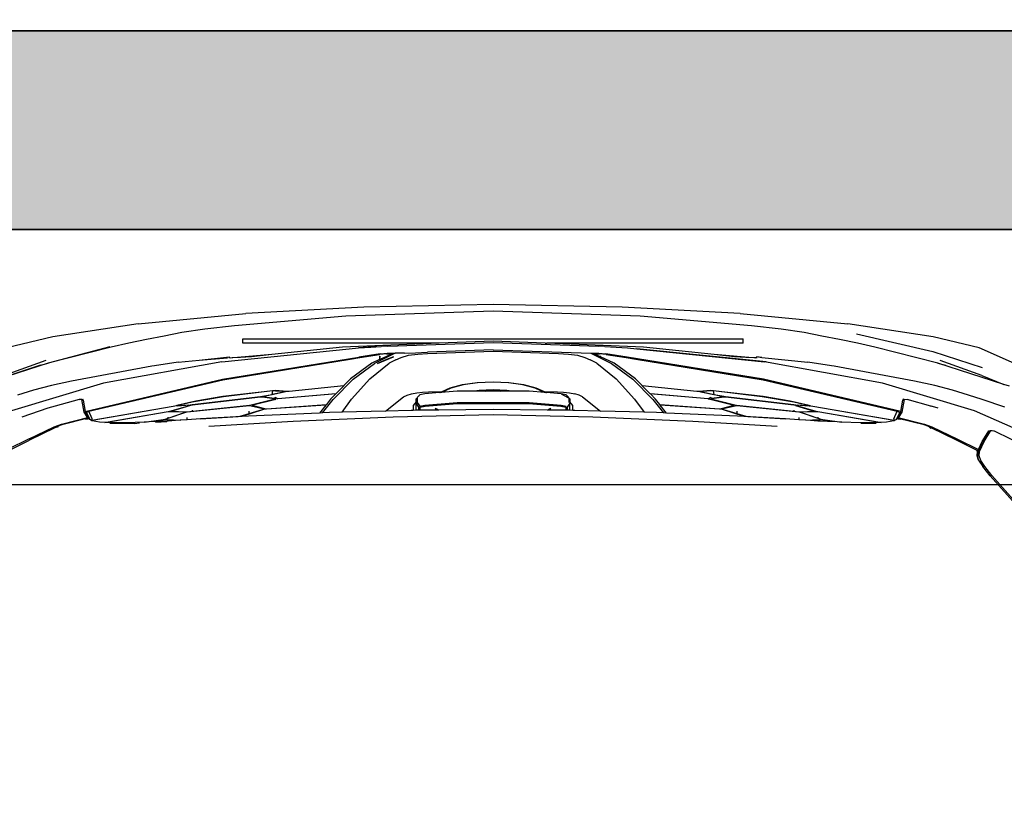
# Model space of a CAD drawing. Units: inches. Extents: x -4737294 to -4736756, y 1716389 to 1717040.
# Tile 14 of 25: x -4737171 to -4737127, y 1716633 to 1716669. Entities that reach past the tile are written whole.
import ezdxf

# ---------------------------------------------------------------- set-up
doc = ezdxf.new("R2010")
doc.units = ezdxf.units.IN
doc.header["$MEASUREMENT"] = 0
for name, color, linetype, lineweight in [('A-ANNO-DIMS', 2, 'Continuous', 18), ('A-EQPM-VEHI', 250, 'Continuous', 13), ('A-WALL-PATT', 244, 'Continuous', 13), ('walls', 252, 'Continuous', 35)]:
    doc.layers.add(name, color=color, linetype=linetype, lineweight=lineweight)
doc.layers.add('Edges', color=250, linetype='Continuous')
doc.styles.get("Standard").update_dxf_attribs({"font": 'arial.ttf'})
doc.dimstyles.get("Standard").update_dxf_attribs({"dimtxt": 8, "dimasz": 0.18, "dimexe": 0.18, "dimexo": 0.0625, "dimgap": 0.09, "dimtad": 0, "dimtih": 1, "dimtoh": 1, "dimzin": 0, "dimdsep": 46, "dimlunit": 3, "dimtxsty": 'Standard', "dimcen": 0.09, "dimadec": 0, "dimazin": 0, "dimtfac": 1, "dimtofl": 0, "dimtmove": 0, "dimatfit": 3, "dimfxl": 1, "dimtolj": 1, "dimtzin": 0, "dimarcsym": 0})

# ---------------------------------------------------------------- blocks, each defined once
blk = doc.blocks.new('Nissan Qashqai pl')
at = {"layer": 'Edges'}
for p, q in [((7.4172, 12.4431), (7.4498, 12.5093)), ((7.5369, 12.5057), (7.4635, 12.4408)), ((7.4638, 12.439), (7.5371, 12.5042)), ((7.4302, 12.4993), (7.3963, 12.4227)), ((7.347, 12.4644), (7.3309, 12.4276)), ((7.3688, 12.4532), (7.3467, 12.3846)), ((7.3596, 12.4302), (7.3688, 12.4532)), ((7.3707, 12.4592), (7.3688, 12.4532)), ((7.3925, 12.4542), (7.3845, 12.4306)), ((7.4167, 12.4393), (7.4169, 12.4406)), ((7.4167, 12.4393), (7.4172, 12.4395)), ((7.417, 12.4377), (7.4167, 12.4393)), ((7.4169, 12.4412), (7.4172, 12.4431)), ((7.4169, 12.4406), (7.4172, 12.4423)), ((7.4169, 12.4406), (7.4169, 12.4412)), ((7.4169, 12.4398), (7.4169, 12.4406)), ((7.4282, 12.4328), (7.4169, 12.4398)), ((7.4172, 12.4395), (7.4169, 12.4398)), ((7.4172, 12.4423), (7.4174, 12.4429)), ((7.4183, 12.4382), (7.4172, 12.4395)), ((7.4175, 12.4429), (7.4174, 12.4429)), ((7.4635, 12.4408), (7.4541, 12.4333)), ((7.4638, 12.439), (7.4541, 12.4313)), ((7.3345, 12.3793), (7.3514, 12.4308)), ((7.3596, 12.4302), (7.344, 12.3869)), ((7.3845, 12.4306), (7.3799, 12.4164)), ((7.4283, 12.4307), (7.417, 12.4377)), ((7.4183, 12.4382), (7.4296, 12.4312)), ((7.4387, 12.428), (7.4282, 12.4328)), ((7.4359, 12.4272), (7.4283, 12.4307)), ((7.4383, 12.4272), (7.4296, 12.4312)), ((7.4479, 12.4293), (7.4431, 12.4276)), ((7.4477, 12.427), (7.4541, 12.4313)), ((7.4541, 12.4333), (7.4479, 12.4293)), ((7.3309, 12.4276), (7.3193, 12.3797)), ((7.3963, 12.4227), (7.3676, 12.3269)), ((7.4255, 12.4044), (7.4367, 12.4268)), ((7.4365, 12.4235), (7.4267, 12.4041)), ((7.4367, 12.4268), (7.4359, 12.4272)), ((7.4378, 12.4261), (7.4365, 12.4235)), ((7.4365, 12.4235), (7.4365, 12.4235)), ((7.4367, 12.4268), (7.4383, 12.4272)), ((7.4379, 12.4263), (7.4378, 12.4261)), ((7.4379, 12.4263), (7.4383, 12.4272)), ((7.4379, 12.4263), (7.4389, 12.4269)), ((7.4384, 12.426), (7.4379, 12.4263)), ((7.4384, 12.426), (7.438, 12.4251)), ((7.4383, 12.4272), (7.4389, 12.4269)), ((7.4389, 12.4269), (7.4384, 12.426)), ((7.4387, 12.4259), (7.4384, 12.426)), ((7.4431, 12.4276), (7.4387, 12.428)), ((7.443, 12.4254), (7.4387, 12.4259)), ((7.44, 12.4264), (7.4389, 12.4269)), ((7.44, 12.4264), (7.4442, 12.4258)), ((7.4477, 12.427), (7.443, 12.4254)), ((7.4442, 12.4258), (7.4477, 12.427)), ((7.3799, 12.4164), (7.375, 12.4)), ((7.375, 12.4), (7.3699, 12.3813)), ((7.4131, 12.3783), (7.4255, 12.4044)), ((7.4267, 12.4041), (7.4139, 12.3778)), ((7.3467, 12.3846), (7.3489, 12.3925)), ((7.3193, 12.3797), (7.3059, 12.291)), ((7.3161, 12.3001), (7.3345, 12.3793)), ((7.3467, 12.3846), (7.33, 12.3192)), ((7.3699, 12.3813), (7.3653, 12.3604)), ((7.3925, 12.3813), (7.3914, 12.3775)), ((7.3937, 12.3851), (7.3925, 12.3813)), ((7.4115, 12.3746), (7.4131, 12.3783)), ((7.4139, 12.3778), (7.4122, 12.3742)), ((7.4133, 12.3759), (7.4142, 12.3776)), ((7.3913, 12.3774), (7.3844, 12.3526)), ((7.3913, 12.3774), (7.3914, 12.3775)), ((7.4033, 12.3435), (7.4101, 12.3708)), ((7.4108, 12.3703), (7.4042, 12.3435)), ((7.4101, 12.3708), (7.4115, 12.3746)), ((7.4122, 12.3742), (7.4108, 12.3703)), ((7.3653, 12.3604), (7.3497, 12.2767)), ((7.3841, 12.3485), (7.3844, 12.3526)), ((7.3846, 12.3495), (7.3841, 12.3485)), ((7.3841, 12.3485), (7.3853, 12.3483)), ((7.3846, 12.3495), (7.3976, 12.347)), ((7.3971, 12.3461), (7.3853, 12.3483)), ((7.3976, 12.347), (7.4026, 12.3439)), ((7.3971, 12.3461), (7.3635, 12.2033)), ((7.364, 12.2029), (7.3968, 12.3424)), ((7.3916, 12.2547), (7.4062, 12.3389)), ((7.4065, 12.3392), (7.3917, 12.2547)), ((7.3968, 12.3424), (7.398, 12.3449)), ((7.4046, 12.3389), (7.3968, 12.3424)), ((7.3983, 12.3458), (7.3971, 12.3461)), ((7.398, 12.3449), (7.3999, 12.344)), ((7.398, 12.3449), (7.4012, 12.3441)), ((7.4012, 12.3441), (7.3983, 12.3458)), ((7.3999, 12.344), (7.4051, 12.3415)), ((7.3999, 12.344), (7.4048, 12.3417)), ((7.4033, 12.3427), (7.4012, 12.3441)), ((7.4012, 12.3441), (7.4015, 12.344)), ((7.4015, 12.344), (7.4028, 12.3437)), ((7.4026, 12.3439), (7.4033, 12.3435)), ((7.4033, 12.3435), (7.4042, 12.3422)), ((7.4042, 12.3422), (7.4033, 12.3427)), ((7.4042, 12.3435), (7.404, 12.3429)), ((7.404, 12.3429), (7.4043, 12.3428)), ((7.404, 12.3429), (7.4043, 12.3425)), ((7.4041, 12.3435), (7.4042, 12.3435)), ((7.4042, 12.3435), (7.4045, 12.3434)), ((7.4042, 12.3422), (7.4043, 12.3425)), ((7.4044, 12.3422), (7.4042, 12.3422)), ((7.4043, 12.3428), (7.4045, 12.3434)), ((7.4043, 12.3428), (7.4046, 12.3425)), ((7.4043, 12.3425), (7.4043, 12.3428)), ((7.4043, 12.3425), (7.4044, 12.3422)), ((7.4044, 12.3422), (7.4046, 12.3419)), ((7.4046, 12.3422), (7.4044, 12.3422)), ((7.4045, 12.3434), (7.405, 12.3456)), ((7.4045, 12.3434), (7.4048, 12.3433)), ((7.4046, 12.3425), (7.4047, 12.3424)), ((7.4047, 12.3424), (7.4046, 12.3422)), ((7.4046, 12.3422), (7.4046, 12.3419)), ((7.4048, 12.3422), (7.4046, 12.3422)), ((7.4046, 12.3419), (7.405, 12.3419)), ((7.4048, 12.3417), (7.4046, 12.3419)), ((7.4046, 12.3389), (7.4062, 12.3389)), ((7.4047, 12.3424), (7.4048, 12.3422)), ((7.4048, 12.3422), (7.405, 12.3419)), ((7.4048, 12.3417), (7.4052, 12.3416)), ((7.4051, 12.3415), (7.4048, 12.3417)), ((7.405, 12.3419), (7.4052, 12.3416)), ((7.4051, 12.3415), (7.4052, 12.3415)), ((7.4052, 12.3416), (7.4052, 12.3415)), ((7.4052, 12.3415), (7.4063, 12.3395)), ((7.4062, 12.3389), (7.4063, 12.3395)), ((7.4063, 12.3395), (7.4065, 12.3392)), ((7.4065, 12.3392), (7.4066, 12.3389)), ((7.4066, 12.3389), (7.408, 12.3313)), ((7.3676, 12.3269), (7.3455, 12.2042)), ((7.408, 12.3313), (7.4083, 12.3258)), ((7.33, 12.3192), (7.3261, 12.3009)), ((7.3971, 12.2599), (7.4083, 12.3258)), ((7.4084, 12.3244), (7.3975, 12.2599)), ((7.4083, 12.3258), (7.4084, 12.3244)), ((7.4084, 12.3244), (7.4087, 12.3195)), ((7.4087, 12.3195), (7.4087, 12.3037)), ((7.4092, 12.3184), (7.4091, 12.3206)), ((7.4092, 12.305), (7.4092, 12.3184)), ((7.3261, 12.3009), (7.3223, 12.2825)), ((7.4087, 12.3037), (7.4081, 12.2848)), ((7.2951, 12.1791), (7.3059, 12.291)), ((7.3223, 12.2825), (7.3186, 12.2641)), ((7.3498, 12.2768), (7.3494, 12.2741)), ((7.3497, 12.2767), (7.3494, 12.2741)), ((7.4054, 12.2651), (7.4081, 12.2848)), ((7.4079, 12.2798), (7.4059, 12.2651)), ((7.4079, 12.2798), (7.4069, 12.2598)), ((7.4081, 12.2838), (7.4079, 12.2798)), ((7.4081, 12.2848), (7.4081, 12.2838)), ((7.3494, 12.2741), (7.3457, 12.2495)), ((7.4049, 12.2631), (7.4054, 12.2651)), ((7.4059, 12.2651), (7.4058, 12.2632)), ((7.3186, 12.2641), (7.3149, 12.2457)), ((7.3908, 12.2366), (7.3965, 12.256)), ((7.391, 12.2387), (7.3967, 12.2579)), ((7.3912, 12.2527), (7.3916, 12.2547)), ((7.3969, 12.257), (7.3965, 12.256)), ((7.3967, 12.2579), (7.3971, 12.2599)), ((7.3968, 12.2559), (7.3969, 12.257)), ((7.3972, 12.2421), (7.3968, 12.2559)), ((7.3975, 12.2599), (7.3973, 12.258)), ((7.3973, 12.258), (7.3977, 12.2439)), ((7.4048, 12.2612), (7.3982, 12.2419)), ((7.3983, 12.244), (7.4038, 12.2599)), ((7.4028, 12.2599), (7.4038, 12.2599)), ((7.4038, 12.2599), (7.4049, 12.2631)), ((7.4053, 12.2622), (7.4048, 12.2612)), ((7.4053, 12.2612), (7.4053, 12.2622)), ((7.4061, 12.2473), (7.4053, 12.2612)), ((7.4059, 12.2618), (7.4056, 12.2621)), ((7.4058, 12.2632), (7.4059, 12.2618)), ((7.4059, 12.2618), (7.4064, 12.2523)), ((7.4069, 12.2598), (7.4064, 12.2523)), ((7.3149, 12.2457), (7.3113, 12.2217)), ((7.3407, 12.2016), (7.3457, 12.2495)), ((7.3909, 12.2508), (7.3864, 12.231)), ((7.3869, 12.2347), (7.3912, 12.2527)), ((7.3901, 12.2368), (7.391, 12.2507)), ((7.3914, 12.2527), (7.3906, 12.2386)), ((7.3911, 12.2518), (7.3909, 12.2508)), ((7.391, 12.2507), (7.3911, 12.2518)), ((7.3912, 12.2517), (7.3911, 12.2518)), ((7.3917, 12.2547), (7.3914, 12.2527)), ((7.4061, 12.2472), (7.4057, 12.24)), ((7.4064, 12.2523), (7.4061, 12.2473)), ((7.4061, 12.2472), (7.4061, 12.2473)), ((7.3813, 12.2021), (7.3869, 12.2347)), ((7.3815, 12.1638), (7.3899, 12.2348)), ((7.3903, 12.2347), (7.382, 12.1639)), ((7.3899, 12.2348), (7.3901, 12.2368)), ((7.3908, 12.2366), (7.3903, 12.2347)), ((7.3905, 12.1754), (7.3966, 12.2347)), ((7.3906, 12.2386), (7.3907, 12.2376)), ((7.3907, 12.2376), (7.391, 12.2387)), ((7.3977, 12.24), (7.3911, 12.1755)), ((7.3957, 12.2348), (7.3966, 12.2348)), ((7.3957, 12.2347), (7.3966, 12.2347)), ((7.3966, 12.2348), (7.3972, 12.24)), ((7.3966, 12.2347), (7.3966, 12.2348)), ((7.3972, 12.24), (7.3972, 12.2421)), ((7.3977, 12.2439), (7.398, 12.2429)), ((7.3982, 12.2419), (7.3977, 12.24)), ((7.398, 12.2429), (7.3983, 12.244)), ((7.4032, 12.24), (7.4057, 12.24)), ((7.4057, 12.24), (7.4048, 12.2262)), ((7.3864, 12.231), (7.3815, 12.2029)), ((7.4022, 12.187), (7.4048, 12.2262)), ((7.4048, 12.2262), (7.4023, 12.1836)), ((7.3113, 12.2217), (7.3078, 12.191)), ((7.4072, 12.1299), (7.4124, 12.2176)), ((7.3455, 12.2062), (7.3317, 12.0717)), ((7.3317, 12.0717), (7.3455, 12.2042)), ((7.3407, 12.2016), (7.34, 12.1962)), ((7.34, 12.1962), (7.3401, 12.1962)), ((7.3401, 12.1962), (7.341, 12.1962)), ((7.3403, 12.1981), (7.3407, 12.2016)), ((7.3635, 12.2033), (7.3405, 12.0616)), ((7.3413, 12.1933), (7.3407, 12.1879)), ((7.341, 12.1962), (7.3414, 12.1962)), ((7.341, 12.1962), (7.341, 12.1962)), ((7.3414, 12.1962), (7.341, 12.1962)), ((7.341, 12.1962), (7.3413, 12.1933)), ((7.3415, 12.1954), (7.3413, 12.1933)), ((7.3413, 12.1933), (7.3413, 12.1931)), ((7.3426, 12.0707), (7.364, 12.2029)), ((7.375, 12.1484), (7.3813, 12.2021)), ((7.3815, 12.2029), (7.3756, 12.1509)), ((7.3078, 12.191), (7.298, 12.075)), ((7.3407, 12.1879), (7.3378, 12.1521)), ((7.341, 12.1848), (7.34, 12.1731)), ((7.3413, 12.1931), (7.341, 12.1848)), ((7.4021, 12.1833), (7.3951, 12.1606)), ((7.399, 12.1756), (7.4017, 12.185)), ((7.4017, 12.185), (7.4022, 12.187)), ((7.4023, 12.1836), (7.4018, 12.1764)), ((7.4023, 12.1836), (7.4021, 12.1833)), ((7.2951, 12.1791), (7.2884, 12.0562)), ((7.3261, 12.1821), (7.3216, 12.1821)), ((7.3216, 11.6621), (7.3216, 12.1821)), ((7.3261, 12.1821), (7.3261, 11.9779)), ((7.34, 12.1731), (7.3378, 12.1521)), ((7.3877, 12.1639), (7.3901, 12.1734)), ((7.3901, 12.1734), (7.3905, 12.1754)), ((7.3911, 12.1755), (7.3913, 12.1737)), ((7.3913, 12.1737), (7.3943, 12.1614)), ((7.3949, 12.1616), (7.399, 12.1756)), ((7.3967, 12.1756), (7.399, 12.1756)), ((7.4018, 12.1764), (7.3986, 12.1025)), ((7.3812, 12.1619), (7.3815, 12.1638)), ((7.382, 12.1639), (7.382, 12.1619)), ((7.3843, 12.1498), (7.3877, 12.1639)), ((7.3903, 12.1716), (7.3844, 12.1479)), ((7.3877, 12.1639), (7.3874, 12.1639)), ((7.3907, 12.1727), (7.3903, 12.1716)), ((7.3909, 12.1716), (7.3907, 12.1727)), ((7.3939, 12.1596), (7.3909, 12.1716)), ((7.3813, 12.1599), (7.3763, 12.1361)), ((7.3792, 12.1518), (7.3812, 12.1619)), ((7.3815, 12.161), (7.3813, 12.1599)), ((7.3817, 12.16), (7.3815, 12.161)), ((7.3832, 12.1493), (7.3817, 12.16)), ((7.382, 12.1619), (7.3838, 12.1497)), ((7.3896, 12.0954), (7.3941, 12.1576)), ((7.3945, 12.1577), (7.3903, 12.0959)), ((7.3941, 12.1576), (7.3939, 12.1596)), ((7.3943, 12.1614), (7.3947, 12.1605)), ((7.3951, 12.1606), (7.3945, 12.1577)), ((7.3947, 12.1605), (7.3949, 12.1616)), ((7.3378, 12.1521), (7.3302, 12.0785)), ((7.376, 12.136), (7.375, 12.1484)), ((7.3756, 12.1509), (7.3792, 12.1518)), ((7.3756, 12.1509), (7.3762, 12.138)), ((7.3764, 12.138), (7.3792, 12.1518)), ((7.3783, 12.0852), (7.3836, 12.1459)), ((7.384, 12.1459), (7.3788, 12.0857)), ((7.3832, 12.1493), (7.3824, 12.1487)), ((7.3824, 12.1487), (7.3832, 12.1492)), ((7.3836, 12.1459), (7.3824, 12.1487)), ((7.3824, 12.1487), (7.3835, 12.1468)), ((7.3838, 12.1497), (7.3832, 12.1493)), ((7.3832, 12.1492), (7.3837, 12.1495)), ((7.3832, 12.1492), (7.3832, 12.1493)), ((7.3836, 12.1459), (7.3835, 12.1468)), ((7.3835, 12.1468), (7.384, 12.1459)), ((7.3837, 12.1495), (7.3843, 12.1498)), ((7.3837, 12.1495), (7.3838, 12.1497)), ((7.384, 12.1459), (7.3842, 12.1495)), ((7.3844, 12.1479), (7.384, 12.1459)), ((7.3842, 12.1495), (7.3843, 12.1498)), ((7.3843, 12.1495), (7.3842, 12.1495)), ((7.3701, 12.0771), (7.3759, 12.1341)), ((7.3761, 12.1341), (7.3704, 12.0773)), ((7.3759, 12.1341), (7.376, 12.136)), ((7.3763, 12.1361), (7.3761, 12.1341)), ((7.3762, 12.137), (7.3764, 12.138)), ((7.3762, 12.138), (7.3762, 12.137)), ((7.3764, 12.1371), (7.3762, 12.137)), ((7.4025, 12.026), (7.4072, 12.1299)), ((7.3986, 12.1025), (7.3903, 12.0959)), ((7.3986, 12.1025), (7.3985, 12.0993)), ((7.3841, 12.091), (7.3788, 12.0857)), ((7.3896, 12.0954), (7.3841, 12.091)), ((7.3845, 12.0883), (7.3985, 12.0993)), ((7.3903, 12.0959), (7.3896, 12.0954)), ((7.3982, 12.092), (7.3978, 12.0791)), ((7.3985, 12.0993), (7.3982, 12.092)), ((7.3633, 12.0674), (7.3845, 12.0883)), ((7.3783, 12.0852), (7.3704, 12.0773)), ((7.3788, 12.0857), (7.3783, 12.0852)), ((7.298, 12.075), (7.2928, 11.9221)), ((7.3302, 12.0785), (7.3261, 11.9779)), ((7.3309, 12.0619), (7.3317, 12.0717)), ((7.341, 12.0605), (7.3426, 12.0707)), ((7.3701, 12.0771), (7.3631, 12.0701)), ((7.3704, 12.0773), (7.3701, 12.0771)), ((7.3842, 12.0693), (7.3978, 12.0791)), ((7.3978, 12.0791), (7.3966, 12.0338)), ((7.3294, 12.0385), (7.3309, 12.0619)), ((7.3405, 12.0616), (7.3369, 12.0394)), ((7.3377, 12.0398), (7.341, 12.0605)), ((7.3631, 12.0701), (7.3469, 12.0481)), ((7.3471, 12.0454), (7.3633, 12.0674)), ((7.363, 12.0501), (7.3842, 12.0693)), ((7.2884, 12.0562), (7.2857, 11.9221)), ((7.3468, 12.0299), (7.363, 12.0501)), ((7.3365, 12.0237), (7.3471, 12.0454)), ((7.3377, 12.0398), (7.3369, 12.0328)), ((7.3469, 12.0481), (7.3402, 12.0337)), ((7.3251, 11.9221), (7.3291, 12.0316)), ((7.3294, 12.0385), (7.3291, 12.0316)), ((7.3362, 12.0248), (7.3365, 12.0321)), ((7.3365, 12.0321), (7.3369, 12.0394)), ((7.3369, 12.0287), (7.3369, 12.0328)), ((7.3402, 12.0337), (7.338, 12.0291)), ((7.3387, 12.0332), (7.3402, 12.0337)), ((7.3468, 12.0299), (7.3432, 12.0231)), ((7.3818, 12.0151), (7.3966, 12.0338)), ((7.3966, 12.0338), (7.3959, 12.0071)), ((7.3329, 11.9221), (7.3365, 12.0237)), ((7.3362, 12.0248), (7.3366, 12.0246)), ((7.3365, 12.0237), (7.3362, 12.0248)), ((7.338, 12.0291), (7.3369, 12.0287)), ((7.3374, 12.0276), (7.3369, 12.0287)), ((7.338, 12.0291), (7.3374, 12.0276)), ((7.3407, 12.0176), (7.3432, 12.0231)), ((7.4002, 11.9221), (7.4025, 12.026)), ((7.3373, 12.0004), (7.3386, 12.01)), ((7.3386, 12.01), (7.3407, 12.0176)), ((7.3801, 12.0115), (7.3786, 12.007)), ((7.3818, 12.0151), (7.3801, 12.0115)), ((7.3367, 11.99), (7.3373, 12.0004)), ((7.3768, 11.9954), (7.3775, 12.0015)), ((7.3775, 12.0015), (7.3786, 12.007)), ((7.3808, 11.9993), (7.3798, 11.9983)), ((7.3807, 11.9991), (7.3798, 11.9983)), ((7.38, 11.9953), (7.383, 12.0011)), ((7.3807, 11.9991), (7.3808, 11.9993)), ((7.381, 11.9993), (7.3807, 11.9991)), ((7.3808, 11.9993), (7.384, 12.0021)), ((7.381, 11.9993), (7.3808, 11.9993)), ((7.383, 12.0011), (7.381, 11.9993)), ((7.3866, 12.0011), (7.383, 12.0011)), ((7.384, 12.0021), (7.387, 12.0021)), ((7.3868, 12.002), (7.3866, 12.0011)), ((7.3875, 12.0011), (7.3866, 12.0011)), ((7.387, 12.0021), (7.3868, 12.002)), ((7.3909, 12.0051), (7.387, 12.0021)), ((7.387, 12.0021), (7.3885, 12.0021)), ((7.3885, 12.0021), (7.3925, 11.9993)), ((7.3955, 12.0021), (7.3885, 12.0021)), ((7.3956, 12.0051), (7.3909, 12.0051)), ((7.3925, 11.9993), (7.3958, 11.9993)), ((7.3925, 11.9993), (7.3929, 11.9981)), ((7.3955, 12.0021), (7.3958, 12.0018)), ((7.3959, 12.0049), (7.3956, 12.0051)), ((7.3959, 12.0051), (7.3956, 12.0051)), ((7.3959, 12.0049), (7.3958, 12.0018)), ((7.3958, 12.0018), (7.3958, 11.9993)), ((7.3958, 11.9993), (7.3958, 11.9981)), ((7.3959, 12.0071), (7.3959, 12.0051)), ((7.3959, 12.0051), (7.3959, 12.0049)), ((7.3343, 11.9221), (7.3367, 11.99)), ((7.3761, 11.9751), (7.3765, 11.989)), ((7.3765, 11.989), (7.3768, 11.9954)), ((7.3787, 11.9928), (7.3774, 11.9778)), ((7.3798, 11.9983), (7.3787, 11.9928)), ((7.3787, 11.9928), (7.38, 11.9953)), ((7.3876, 11.9595), (7.3904, 11.9928)), ((7.3917, 11.9926), (7.3889, 11.9594)), ((7.3904, 11.9928), (7.3916, 11.9983)), ((7.3929, 11.9981), (7.3917, 11.9926)), ((7.3958, 11.9981), (7.3929, 11.9981)), ((7.3958, 11.9981), (7.3956, 11.9801)), ((7.3938, 11.9823), (7.3956, 11.9801)), ((7.3956, 11.9788), (7.3938, 11.981)), ((7.3956, 11.9788), (7.3951, 11.9221)), ((7.3956, 11.9801), (7.3956, 11.9788)), ((7.3261, 11.9764), (7.3238, 11.9221)), ((7.3261, 11.9764), (7.3261, 11.9779)), ((7.3724, 11.9667), (7.3761, 11.9751)), ((7.3771, 11.9757), (7.3727, 11.9658)), ((7.3773, 11.9759), (7.3759, 11.9595)), ((7.3761, 11.9751), (7.3769, 11.9767)), ((7.3769, 11.9767), (7.3771, 11.977)), ((7.3774, 11.9778), (7.3771, 11.9771)), ((7.3771, 11.9771), (7.3774, 11.9774)), ((7.3771, 11.9771), (7.3771, 11.977)), ((7.3773, 11.9759), (7.3771, 11.9757)), ((7.3774, 11.9774), (7.3773, 11.9759)), ((7.3774, 11.9774), (7.3774, 11.9778)), ((7.369, 11.9536), (7.3724, 11.9667)), ((7.3727, 11.9658), (7.3693, 11.953)), ((7.3759, 11.9595), (7.3759, 11.9417)), ((7.3876, 11.8847), (7.3876, 11.9595)), ((7.3889, 11.9594), (7.3889, 11.8848)), ((7.3668, 11.9384), (7.369, 11.9536)), ((7.3693, 11.953), (7.3672, 11.9381)), ((7.3661, 11.9221), (7.3668, 11.9384)), ((7.3672, 11.9381), (7.3665, 11.9221)), ((7.3759, 11.9417), (7.3751, 11.9363)), ((7.3759, 11.9417), (7.3759, 11.9303)), ((7.3751, 11.9363), (7.3745, 11.9221)), ((7.3755, 11.9221), (7.3759, 11.9303)), ((7.3759, 11.9303), (7.3759, 11.9139)), ((7.2857, 11.9221), (7.2884, 11.7879)), ((7.2928, 11.9221), (7.298, 11.7692)), ((7.3238, 11.9221), (7.3261, 11.8662)), ((7.3291, 11.8126), (7.3251, 11.9221)), ((7.3329, 11.9221), (7.3354, 11.8539)), ((7.3367, 11.8541), (7.3343, 11.9221)), ((7.3668, 11.9057), (7.3661, 11.9221)), ((7.3665, 11.9221), (7.3672, 11.9061)), ((7.3745, 11.9221), (7.3751, 11.9078)), ((7.3759, 11.9139), (7.3755, 11.9221)), ((7.3951, 11.9221), (7.3956, 11.8653)), ((7.4025, 11.8181), (7.4002, 11.9221)), ((7.3751, 11.9078), (7.3759, 11.9025)), ((7.3759, 11.9139), (7.3759, 11.9025)), ((7.369, 11.8905), (7.3668, 11.9057)), ((7.3672, 11.9061), (7.3693, 11.8911)), ((7.3759, 11.9025), (7.3759, 11.8847)), ((7.3724, 11.8775), (7.369, 11.8905)), ((7.3693, 11.8911), (7.3727, 11.8783)), ((7.3761, 11.8691), (7.3724, 11.8775)), ((7.3727, 11.8783), (7.3771, 11.8685)), ((7.3759, 11.8847), (7.3773, 11.8682)), ((7.3904, 11.8513), (7.3876, 11.8847)), ((7.3889, 11.8848), (7.3917, 11.8516)), ((7.3261, 11.8662), (7.3302, 11.7656)), ((7.3261, 11.8662), (7.3261, 11.6621)), ((7.3765, 11.8551), (7.3761, 11.8691)), ((7.3769, 11.8674), (7.3761, 11.8691)), ((7.3771, 11.8671), (7.3769, 11.8674)), ((7.3771, 11.8685), (7.3773, 11.8682)), ((7.3771, 11.8671), (7.3771, 11.8671)), ((7.3771, 11.8671), (7.3774, 11.8664)), ((7.3774, 11.8668), (7.3771, 11.8671)), ((7.3773, 11.8682), (7.3774, 11.8668)), ((7.3774, 11.8668), (7.3774, 11.8664)), ((7.3774, 11.8664), (7.3787, 11.8513)), ((7.3938, 11.8632), (7.3956, 11.8653)), ((7.3956, 11.864), (7.3938, 11.8619)), ((7.3956, 11.8653), (7.3956, 11.864)), ((7.3956, 11.864), (7.3958, 11.8461)), ((7.3361, 11.8416), (7.3354, 11.8539)), ((7.3373, 11.8438), (7.3367, 11.8541)), ((7.3768, 11.8488), (7.3765, 11.8551)), ((7.3775, 11.8427), (7.3768, 11.8488)), ((7.3787, 11.8513), (7.3798, 11.8459)), ((7.3798, 11.8459), (7.3808, 11.8448)), ((7.3875, 11.8431), (7.3916, 11.8459)), ((7.3916, 11.8459), (7.3904, 11.8513)), ((7.3917, 11.8516), (7.3929, 11.8461)), ((7.3929, 11.8461), (7.3925, 11.8448)), ((7.3929, 11.8461), (7.3958, 11.8461)), ((7.3958, 11.8461), (7.3958, 11.8448)), ((7.3362, 11.8301), (7.3361, 11.8416)), ((7.3386, 11.8342), (7.3373, 11.8438)), ((7.3786, 11.8372), (7.3775, 11.8427)), ((7.3801, 11.8327), (7.3786, 11.8372)), ((7.3808, 11.8448), (7.3807, 11.8451)), ((7.3808, 11.8448), (7.381, 11.8448)), ((7.384, 11.8421), (7.3808, 11.8448)), ((7.383, 11.8431), (7.3875, 11.8431)), ((7.387, 11.8421), (7.384, 11.8421)), ((7.387, 11.8421), (7.3909, 11.8391)), ((7.3885, 11.8421), (7.387, 11.8421)), ((7.3925, 11.8448), (7.3885, 11.8421)), ((7.3955, 11.8421), (7.3885, 11.8421)), ((7.3909, 11.8391), (7.3956, 11.8391)), ((7.3958, 11.8448), (7.3925, 11.8448)), ((7.3958, 11.8423), (7.3955, 11.8421)), ((7.3956, 11.8391), (7.3959, 11.8392)), ((7.3956, 11.8391), (7.3959, 11.8391)), ((7.3958, 11.8448), (7.3958, 11.8423)), ((7.3958, 11.8423), (7.3959, 11.8392)), ((7.3959, 11.8392), (7.3959, 11.8391)), ((7.3959, 11.8391), (7.3959, 11.8371)), ((7.3959, 11.8371), (7.3966, 11.8103)), ((7.3362, 11.8301), (7.3365, 11.8204)), ((7.3407, 11.8266), (7.3386, 11.8342)), ((7.3432, 11.821), (7.3407, 11.8266)), ((7.3818, 11.8291), (7.3801, 11.8327)), ((7.3966, 11.8103), (7.3818, 11.8291)), ((7.3362, 11.8194), (7.3365, 11.8204)), ((7.3367, 11.8196), (7.3362, 11.8194)), ((7.3365, 11.812), (7.3362, 11.8194)), ((7.3365, 11.8204), (7.3471, 11.7987)), ((7.3369, 11.8155), (7.3374, 11.8165)), ((7.3369, 11.8113), (7.3369, 11.8155)), ((7.3369, 11.8155), (7.338, 11.8151)), ((7.3374, 11.8165), (7.338, 11.8151)), ((7.338, 11.8151), (7.343, 11.8045)), ((7.3401, 11.8186), (7.3431, 11.8112)), ((7.347, 11.8021), (7.3401, 11.8186)), ((7.3432, 11.821), (7.3468, 11.8142)), ((7.4072, 11.7142), (7.4025, 11.8181)), ((7.3291, 11.8126), (7.3294, 11.8057)), ((7.3301, 11.7949), (7.3294, 11.8057)), ((7.3369, 11.8047), (7.3365, 11.812)), ((7.3369, 11.8113), (7.3377, 11.8044)), ((7.3369, 11.8047), (7.3405, 11.7825)), ((7.3377, 11.8042), (7.3377, 11.8044)), ((7.343, 11.8045), (7.3396, 11.8043)), ((7.3396, 11.8043), (7.3431, 11.8042)), ((7.343, 11.8045), (7.3431, 11.8042)), ((7.3431, 11.8112), (7.347, 11.8021)), ((7.363, 11.794), (7.3468, 11.8142)), ((7.3966, 11.8103), (7.3978, 11.7651)), ((7.3295, 11.8012), (7.3309, 11.7822)), ((7.3295, 11.8012), (7.3301, 11.7949)), ((7.3309, 11.7822), (7.3301, 11.7949)), ((7.341, 11.7837), (7.3377, 11.8042)), ((7.3431, 11.8042), (7.3469, 11.7961)), ((7.3469, 11.7961), (7.3631, 11.774)), ((7.3633, 11.7767), (7.3471, 11.7987)), ((7.3842, 11.7749), (7.363, 11.794)), ((7.2884, 11.7879), (7.2951, 11.6651)), ((7.3317, 11.7724), (7.3309, 11.7822)), ((7.3635, 11.6409), (7.3405, 11.7825)), ((7.3426, 11.7735), (7.341, 11.7837)), ((7.3631, 11.774), (7.3701, 11.7671)), ((7.3845, 11.7558), (7.3633, 11.7767)), ((7.3978, 11.7651), (7.3842, 11.7749)), ((7.298, 11.7692), (7.3078, 11.6532)), ((7.3302, 11.7656), (7.3378, 11.6921)), ((7.3455, 11.64), (7.3317, 11.7724)), ((7.364, 11.6413), (7.3426, 11.7735)), ((7.3759, 11.7101), (7.3701, 11.7671)), ((7.3701, 11.7671), (7.3704, 11.7668)), ((7.3704, 11.7668), (7.3761, 11.71)), ((7.3704, 11.7668), (7.3783, 11.759)), ((7.3978, 11.7651), (7.3982, 11.7521)), ((7.3836, 11.6983), (7.3783, 11.759)), ((7.3783, 11.759), (7.3788, 11.7585)), ((7.3788, 11.7585), (7.384, 11.6982)), ((7.3788, 11.7585), (7.3841, 11.7532)), ((7.3841, 11.7532), (7.3896, 11.7488)), ((7.3985, 11.7448), (7.3845, 11.7558)), ((7.3941, 11.6865), (7.3896, 11.7488)), ((7.3896, 11.7488), (7.3903, 11.7483)), ((7.3903, 11.7483), (7.3945, 11.6865)), ((7.3903, 11.7483), (7.3986, 11.7417)), ((7.3982, 11.7521), (7.3985, 11.7448)), ((7.3985, 11.7448), (7.3986, 11.7417)), ((7.3986, 11.7417), (7.4018, 11.6678)), ((7.4124, 11.6265), (7.4072, 11.7142)), ((7.375, 11.6957), (7.376, 11.7081)), ((7.3762, 11.7062), (7.3757, 11.6959)), ((7.376, 11.7081), (7.3759, 11.7101)), ((7.3761, 11.71), (7.3763, 11.7081)), ((7.3762, 11.7062), (7.3764, 11.7061)), ((7.3763, 11.7081), (7.3813, 11.6842)), ((7.3764, 11.7061), (7.3792, 11.6924)), ((7.3378, 11.6921), (7.3407, 11.6563)), ((7.3378, 11.6921), (7.34, 11.671)), ((7.3813, 11.642), (7.375, 11.6957)), ((7.3757, 11.6959), (7.3756, 11.6933)), ((7.3792, 11.6924), (7.3756, 11.6933)), ((7.3756, 11.6933), (7.3815, 11.6413)), ((7.3757, 11.6959), (7.3757, 11.6959)), ((7.3812, 11.6823), (7.3792, 11.6924)), ((7.3817, 11.6844), (7.3832, 11.6949)), ((7.3838, 11.6944), (7.382, 11.6823)), ((7.3824, 11.6955), (7.3836, 11.6983)), ((7.3835, 11.6973), (7.3824, 11.6955)), ((7.3834, 11.6959), (7.3824, 11.6955)), ((7.3824, 11.6955), (7.3832, 11.6949)), ((7.3832, 11.695), (7.3824, 11.6955)), ((7.3832, 11.695), (7.3834, 11.6959)), ((7.3838, 11.6947), (7.3832, 11.695)), ((7.3832, 11.6949), (7.3838, 11.6944)), ((7.3837, 11.696), (7.3834, 11.6959)), ((7.3835, 11.6973), (7.3836, 11.6983)), ((7.3836, 11.6975), (7.3835, 11.6973)), ((7.3836, 11.6975), (7.3836, 11.6983)), ((7.384, 11.6982), (7.3836, 11.6975)), ((7.3844, 11.6963), (7.3837, 11.696)), ((7.3838, 11.6947), (7.3837, 11.696)), ((7.3843, 11.6944), (7.3838, 11.6947)), ((7.3843, 11.6942), (7.3838, 11.6944)), ((7.3843, 11.6944), (7.3844, 11.6963)), ((7.3843, 11.6942), (7.3843, 11.6944)), ((7.3877, 11.6803), (7.3843, 11.6942)), ((7.3844, 11.6963), (7.3903, 11.6725)), ((7.3815, 11.6804), (7.3812, 11.6823)), ((7.3813, 11.6842), (7.3817, 11.6844)), ((7.3817, 11.6841), (7.3813, 11.6842)), ((7.3817, 11.6841), (7.3817, 11.6844)), ((7.382, 11.6823), (7.382, 11.6803)), ((7.3909, 11.6728), (7.3939, 11.6846)), ((7.3943, 11.6827), (7.3913, 11.6705)), ((7.3939, 11.6846), (7.3941, 11.6865)), ((7.3943, 11.6827), (7.3949, 11.6826)), ((7.3943, 11.6827), (7.395, 11.6825)), ((7.3945, 11.6865), (7.3951, 11.6835)), ((7.395, 11.6825), (7.3949, 11.6826)), ((7.399, 11.6686), (7.395, 11.6825)), ((7.3951, 11.6835), (7.4021, 11.6609)), ((7.3899, 11.6094), (7.3815, 11.6804)), ((7.382, 11.6803), (7.3903, 11.6095)), ((7.3874, 11.6803), (7.3877, 11.6803)), ((7.3901, 11.6707), (7.3877, 11.6803)), ((7.3909, 11.6728), (7.3903, 11.6725)), ((7.3909, 11.6725), (7.3903, 11.6725)), ((7.3909, 11.6725), (7.3909, 11.6728)), ((7.3059, 11.5532), (7.2951, 11.6651)), ((7.3261, 11.6621), (7.3216, 11.6621)), ((7.34, 11.671), (7.341, 11.6594)), ((7.3905, 11.6687), (7.3901, 11.6707)), ((7.3966, 11.6095), (7.3905, 11.6687)), ((7.3913, 11.6705), (7.3911, 11.6687)), ((7.3911, 11.6687), (7.3977, 11.6042)), ((7.399, 11.6686), (7.3967, 11.6686)), ((7.4017, 11.6592), (7.399, 11.6686)), ((7.4018, 11.6678), (7.4022, 11.6609)), ((7.4022, 11.6609), (7.4021, 11.6609)), ((7.4022, 11.6609), (7.4022, 11.6609)), ((7.3078, 11.6532), (7.3113, 11.6224)), ((7.3407, 11.6563), (7.3413, 11.6509)), ((7.341, 11.6594), (7.3413, 11.6511)), ((7.341, 11.648), (7.3413, 11.6509)), ((7.3413, 11.6511), (7.3413, 11.6509)), ((7.3413, 11.6509), (7.3415, 11.6488)), ((7.4022, 11.6571), (7.4017, 11.6592)), ((7.4022, 11.6609), (7.4021, 11.6609)), ((7.4022, 11.6609), (7.4048, 11.618)), ((7.4048, 11.618), (7.4022, 11.6571)), ((7.3401, 11.648), (7.34, 11.648)), ((7.3438, 11.6167), (7.34, 11.648)), ((7.341, 11.648), (7.3401, 11.648)), ((7.3414, 11.648), (7.341, 11.648)), ((7.341, 11.648), (7.3414, 11.648)), ((7.3438, 11.6167), (7.3412, 11.646)), ((7.3971, 11.4981), (7.3635, 11.6409)), ((7.3968, 11.5018), (7.364, 11.6413)), ((7.3869, 11.6094), (7.3813, 11.642)), ((7.3815, 11.6413), (7.3864, 11.6131)), ((7.3455, 11.64), (7.3676, 11.5172)), ((7.3113, 11.6224), (7.3149, 11.5984)), ((7.3457, 11.5947), (7.3438, 11.6167)), ((7.3864, 11.6131), (7.3909, 11.5933)), ((7.4048, 11.618), (7.4057, 11.6042)), ((7.3912, 11.5914), (7.3869, 11.6094)), ((7.3901, 11.6073), (7.3899, 11.6094)), ((7.391, 11.5935), (7.3901, 11.6073)), ((7.3903, 11.6095), (7.3908, 11.6076)), ((7.3906, 11.6055), (7.391, 11.6055)), ((7.3906, 11.6055), (7.391, 11.6054)), ((7.3906, 11.6055), (7.3914, 11.5914)), ((7.3908, 11.6076), (7.3965, 11.5881)), ((7.391, 11.6054), (7.391, 11.6055)), ((7.3967, 11.5862), (7.391, 11.6054)), ((7.3966, 11.6095), (7.3957, 11.6095)), ((7.3972, 11.6042), (7.3966, 11.6095)), ((7.3968, 11.5882), (7.3972, 11.6021)), ((7.3972, 11.6021), (7.3972, 11.6042)), ((7.3977, 11.6003), (7.3973, 11.5862)), ((7.3977, 11.6042), (7.3982, 11.6022)), ((7.3977, 11.6003), (7.3983, 11.6002)), ((7.3977, 11.6003), (7.3983, 11.6001)), ((7.3982, 11.6022), (7.4048, 11.5829)), ((7.3983, 11.6001), (7.3983, 11.6002)), ((7.4038, 11.5843), (7.3983, 11.6001)), ((7.4057, 11.6042), (7.4032, 11.6042)), ((7.4057, 11.6042), (7.4061, 11.597)), ((7.3149, 11.5984), (7.3186, 11.58)), ((7.3457, 11.5947), (7.3494, 11.57)), ((7.391, 11.5935), (7.3909, 11.5933)), ((7.391, 11.5934), (7.3909, 11.5933)), ((7.3916, 11.5894), (7.3912, 11.5914)), ((7.3914, 11.5914), (7.3917, 11.5895)), ((7.4062, 11.5053), (7.3916, 11.5894)), ((7.3917, 11.5895), (7.4065, 11.505)), ((7.4053, 11.5831), (7.4061, 11.5969)), ((7.4064, 11.5919), (7.406, 11.5834)), ((7.4061, 11.5969), (7.4061, 11.597)), ((7.4061, 11.5969), (7.4064, 11.5919)), ((7.4064, 11.5919), (7.4069, 11.5844)), ((7.3186, 11.58), (7.3223, 11.5616)), ((7.3968, 11.5882), (7.3965, 11.5881)), ((7.3971, 11.5842), (7.3967, 11.5862)), ((7.3968, 11.5882), (7.3973, 11.5884)), ((7.4083, 11.5184), (7.3971, 11.5842)), ((7.3973, 11.5862), (7.3975, 11.5843)), ((7.3975, 11.5843), (7.4084, 11.5198)), ((7.4038, 11.5843), (7.4028, 11.5843)), ((7.4049, 11.5811), (7.4038, 11.5843)), ((7.4053, 11.5831), (7.4048, 11.5829)), ((7.4053, 11.583), (7.4048, 11.5829)), ((7.4054, 11.5791), (7.4049, 11.5811)), ((7.406, 11.5834), (7.4053, 11.5831)), ((7.406, 11.5833), (7.4053, 11.583)), ((7.4053, 11.583), (7.4053, 11.5831)), ((7.4081, 11.5593), (7.4054, 11.5791)), ((7.406, 11.5833), (7.4058, 11.581)), ((7.4058, 11.581), (7.4059, 11.579)), ((7.4059, 11.579), (7.4079, 11.5644)), ((7.406, 11.5834), (7.406, 11.5833)), ((7.4069, 11.5844), (7.4079, 11.5644)), ((7.4081, 11.5711), (7.4075, 11.5828)), ((7.3494, 11.57), (7.3497, 11.5674)), ((7.3494, 11.57), (7.3498, 11.5674)), ((7.3223, 11.5616), (7.3261, 11.5433)), ((7.3497, 11.5674), (7.3653, 11.4838)), ((7.4079, 11.5644), (7.4081, 11.5604)), ((7.4079, 11.5644), (7.4081, 11.5629)), ((7.4081, 11.5604), (7.4081, 11.5593)), ((7.4081, 11.5593), (7.4087, 11.5405)), ((7.3059, 11.5532), (7.3193, 11.4645)), ((7.4092, 11.5416), (7.409, 11.5485)), ((7.4096, 11.549), (7.4092, 11.5521)), ((7.4093, 11.5546), (7.4095, 11.5529)), ((7.3261, 11.5433), (7.33, 11.5249)), ((7.4087, 11.5405), (7.4087, 11.5246)), ((7.4092, 11.5258), (7.4092, 11.5416)), ((7.3297, 11.5237), (7.3467, 11.4596)), ((7.33, 11.5249), (7.3467, 11.4596)), ((7.4083, 11.5184), (7.408, 11.5129)), ((7.4084, 11.5198), (7.4083, 11.5184)), ((7.4087, 11.5246), (7.4084, 11.5198)), ((7.4091, 11.5235), (7.4092, 11.5258)), ((7.3676, 11.5172), (7.3963, 11.4215)), ((7.408, 11.5129), (7.4066, 11.5052)), ((7.3976, 11.4971), (7.3846, 11.4946)), ((7.3853, 11.4958), (7.3971, 11.4981)), ((7.4046, 11.5053), (7.3968, 11.5018)), ((7.398, 11.4993), (7.3968, 11.5018)), ((7.3971, 11.4981), (7.3983, 11.4983)), ((7.4026, 11.5002), (7.3976, 11.4971)), ((7.398, 11.4993), (7.4048, 11.5024)), ((7.4012, 11.5001), (7.398, 11.4993)), ((7.3983, 11.4983), (7.4012, 11.5001)), ((7.4012, 11.5001), (7.4033, 11.5014)), ((7.403, 11.5005), (7.4026, 11.5002)), ((7.403, 11.5005), (7.4028, 11.5004)), ((7.4033, 11.5007), (7.403, 11.5005)), ((7.4033, 11.5014), (7.4042, 11.502)), ((7.4042, 11.502), (7.4033, 11.5007)), ((7.4033, 11.5005), (7.4033, 11.5007)), ((7.4034, 11.5005), (7.4033, 11.5005)), ((7.4101, 11.4733), (7.4033, 11.5005)), ((7.4043, 11.5016), (7.404, 11.5012)), ((7.4043, 11.5014), (7.404, 11.5012)), ((7.404, 11.5012), (7.4108, 11.4738)), ((7.4042, 11.502), (7.4044, 11.502)), ((7.4043, 11.5016), (7.4042, 11.502)), ((7.4044, 11.502), (7.4043, 11.5016)), ((7.4046, 11.5016), (7.4043, 11.5014)), ((7.4043, 11.5014), (7.4043, 11.5016)), ((7.4045, 11.5008), (7.4043, 11.5014)), ((7.4046, 11.5023), (7.4044, 11.502)), ((7.4044, 11.502), (7.4046, 11.502)), ((7.4048, 11.5008), (7.4045, 11.5008)), ((7.405, 11.4985), (7.4045, 11.5008)), ((7.4062, 11.5053), (7.4046, 11.5053)), ((7.4046, 11.5023), (7.4048, 11.5024)), ((7.405, 11.5023), (7.4046, 11.5023)), ((7.4046, 11.5023), (7.4046, 11.502)), ((7.4046, 11.502), (7.4047, 11.5018)), ((7.4046, 11.502), (7.4048, 11.502)), ((7.4047, 11.5018), (7.4046, 11.5016)), ((7.4048, 11.502), (7.4047, 11.5018)), ((7.4048, 11.5024), (7.4052, 11.5027)), ((7.4052, 11.5026), (7.4048, 11.5024)), ((7.405, 11.5023), (7.4048, 11.502)), ((7.4052, 11.5026), (7.405, 11.5023)), ((7.4063, 11.5047), (7.4052, 11.5027)), ((7.4052, 11.5027), (7.4052, 11.5026)), ((7.4063, 11.5047), (7.4062, 11.5053)), ((7.4065, 11.505), (7.4063, 11.5047)), ((7.4066, 11.5052), (7.4065, 11.505)), ((7.3853, 11.4958), (7.3841, 11.4956)), ((7.3844, 11.4916), (7.3841, 11.4956)), ((7.3846, 11.4946), (7.3844, 11.4916)), ((7.3844, 11.4916), (7.3914, 11.4667)), ((7.3853, 11.4958), (7.3846, 11.4946)), ((7.3653, 11.4838), (7.3699, 11.4629)), ((7.3914, 11.4667), (7.3925, 11.4629)), ((7.4115, 11.4695), (7.4101, 11.4733)), ((7.4108, 11.4738), (7.4122, 11.47)), ((7.4131, 11.4659), (7.4115, 11.4695)), ((7.4122, 11.47), (7.4139, 11.4664)), ((7.4126, 11.47), (7.4125, 11.4702)), ((7.4132, 11.4685), (7.4126, 11.47)), ((7.3193, 11.4645), (7.3309, 11.4166)), ((7.344, 11.4572), (7.3596, 11.4139)), ((7.3489, 11.4517), (7.3467, 11.4596)), ((7.3467, 11.4596), (7.3686, 11.3913)), ((7.3699, 11.4629), (7.375, 11.4442)), ((7.3925, 11.4629), (7.3937, 11.4591)), ((7.3937, 11.4591), (7.4029, 11.4321)), ((7.4255, 11.4398), (7.4131, 11.4659)), ((7.4139, 11.4664), (7.4267, 11.4401)), ((7.3489, 11.4517), (7.3686, 11.3913)), ((7.375, 11.4442), (7.3799, 11.4278)), ((7.4255, 11.4398), (7.4367, 11.4174)), ((7.4379, 11.4179), (7.4267, 11.4401))]:
    blk.add_line(p, q, dxfattribs=at)
blk = doc.blocks.new('car')
blk.add_blockref('Nissan Qashqai pl', (-9.7433, -11.9151))
blk = doc.blocks.new('*D63')
at = {"layer": 'A-ANNO-DIMS', "color": 0, "lineweight": -2, "transparency": 16777216}
for p, q in [((-4737062.207, 1716647.493), (-4737270.324, 1716647.493)), ((-4737270.144, 1716647.313), (-4737270.144, 1716628.418)), ((-4737270.144, 1716601.064), (-4737270.144, 1716619.959)), ((-4737062.207, 1716600.884), (-4737270.324, 1716600.884))]:
    blk.add_line(p, q, dxfattribs=at)
at = {"layer": 'A-ANNO-DIMS', "color": 0, "transparency": 16777216}
for points in [[(-4737270.174, 1716647.313), (-4737270.114, 1716647.313), (-4737270.144, 1716647.493)], [(-4737270.174, 1716601.064), (-4737270.114, 1716601.064), (-4737270.144, 1716600.884)]]:
    blk.add_solid(points, dxfattribs=at)
at = {"layer": 'Defpoints', "color": 0, "transparency": 16777216}
for p in [(-4737270.144, 1716647.493), (-4737062.144, 1716647.493), (-4737062.144, 1716600.884)]:
    blk.add_point(p, dxfattribs=at)
at = {"layer": 'A-ANNO-DIMS', "color": 0, "transparency": 16777216, "insert": (-4737270.144, 1716624.188), "char_height": 8, "attachment_point": 5}
blk.add_mtext('\\A1;3\'-10 1/2"', dxfattribs=at)

msp = doc.modelspace()

# ---------------------------------------------------------------- hatches: boundary and pattern name
at = {"layer": 'A-WALL-PATT'}
h = msp.add_hatch(color=256, dxfattribs=at)
h.dxf.hatch_style = 1
h.paths.add_polyline_path([(-4737206.144, 1716844.565), (-4737110.144, 1716844.565), (-4737110.144, 1716823.907), (-4737105.644, 1716823.907), (-4737105.644, 1716844.565), (-4737098.44, 1716844.565), (-4737098.44, 1716849.065), (-4737206.144, 1716849.065), (-4737206.144, 1716993.065), (-4736864.144, 1716993.065), (-4736864.144, 1716849.065), (-4736963.275, 1716849.065), (-4736994.446, 1716849.065), (-4736997.144, 1716849.065), (-4736997.144, 1716844.565), (-4736864.144, 1716844.565), (-4736864.144, 1716668.565), (-4736934.391, 1716668.565), (-4736934.391, 1716664.065), (-4736864.144, 1716664.065), (-4736864.144, 1716462.065), (-4736855.144, 1716462.065), (-4736855.144, 1717002.065), (-4737215.144, 1717002.065), (-4737215.144, 1716462.065), (-4737206.144, 1716462.065), (-4737206.144, 1716659.065), (-4737062.144, 1716659.065), (-4737062.144, 1716647.493), (-4737057.644, 1716647.493), (-4737057.644, 1716796.565), (-4737071.812, 1716796.565), (-4737071.812, 1716792.065), (-4737070.805, 1716792.065), (-4737062.144, 1716792.065), (-4737062.144, 1716668.065), (-4737206.144, 1716668.065), (-4737206.144, 1716792.065), (-4737093.784, 1716792.065), (-4737093.784, 1716796.565), (-4737206.144, 1716796.565)])

# ---------------------------------------------------------------- linework, layer by layer
at = {"layer": 'walls'}
for p, q in [((-4737206.144, 1716668.065), (-4737062.144, 1716668.065)), ((-4737206.144, 1716659.065), (-4737062.144, 1716659.065))]:
    msp.add_line(p, q, dxfattribs=at)

# ---------------------------------------------------------------- block references
at = {"layer": 'A-EQPM-VEHI', "xscale": 43.56002006885659, "yscale": 43.56002006885659, "zscale": 43.56002006885659, "rotation": 270}
msp.add_blockref('car', (-4737150.017, 1716548.61), dxfattribs=at)

# ---------------------------------------------------------------- dimensions: what is measured, and where the dimension line sits
at = {"layer": 'A-ANNO-DIMS'}
dim = msp.add_linear_dim(base=(-4737270.144, 1716647.493), p1=(-4737062.144, 1716600.884), p2=(-4737062.144, 1716647.493), angle=90, dimstyle='Standard', override={"dimdec": 1, "dimlfac": 1, "dimrnd": 0, "dimzin": 1, "dimdsep": 46, "dimlunit": 4, "dimfrac": 2}, dxfattribs=at)
dim.commit()
dim.dimension.update_dxf_attribs({"geometry": '*D63', "text_midpoint": (-4737270.144, 1716624.188)})

doc.saveas('drawing.dxf')
